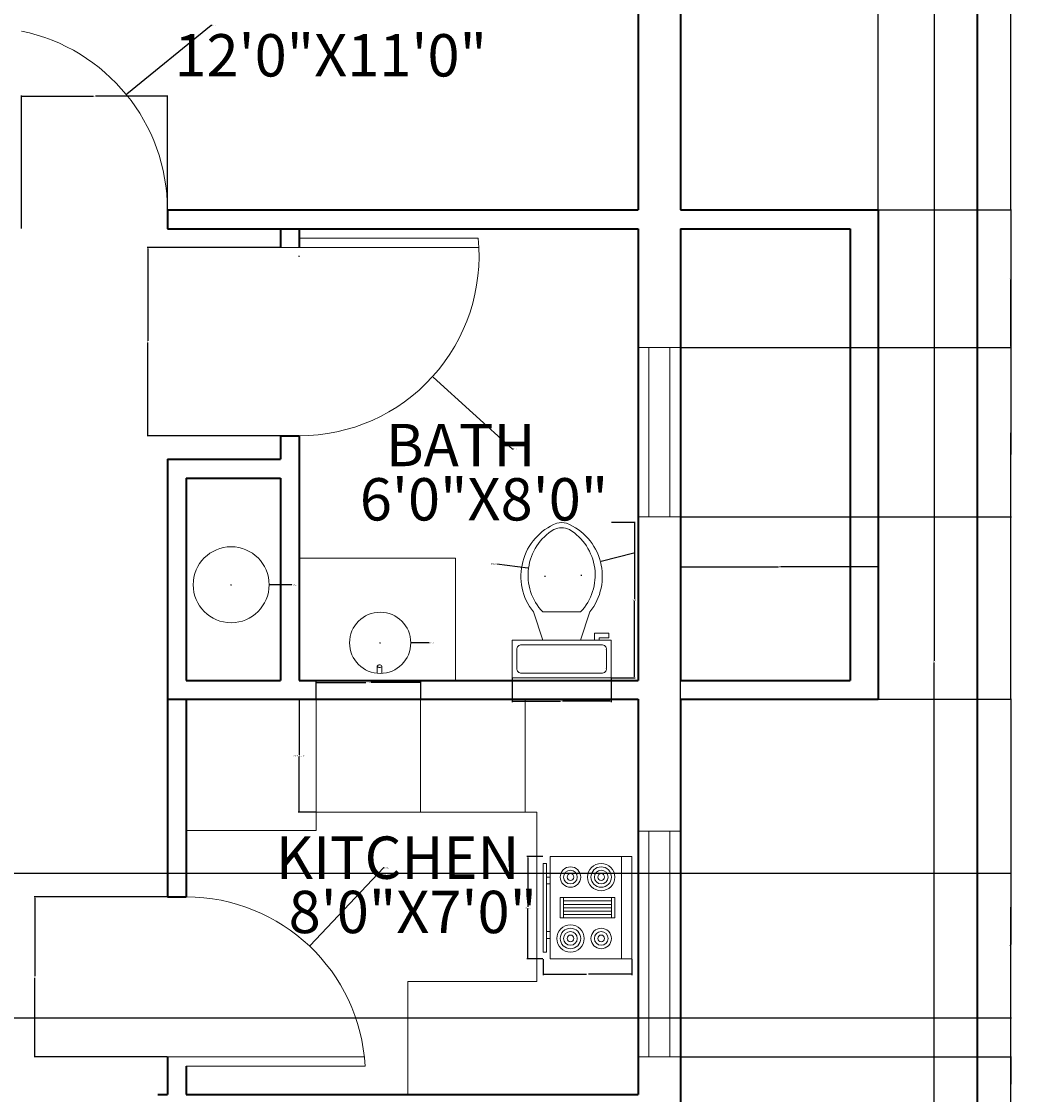
# Model space of a CAD drawing. Units: inches. Extents: x 1762 to 3150, y 1680 to 2382.
# Tile 3 of 6: x 1983 to 2199, y 1904 to 2132. Entities that reach past the tile are written whole.
import ezdxf

# ---------------------------------------------------------------- set-up
doc = ezdxf.new("R2010")
doc.units = ezdxf.units.IN
for name, color, linetype, lineweight in [('A-ANNO-DIMS', 2, 'Continuous', 18), ('A-ANNO-TTLB', 7, 'Continuous', 35), ('A-AREA-IDEN', 7, 'Continuous', 18), ('A-DOOR', 3, 'Continuous', 18), ('A-EQPM', 8, 'Continuous', 18), ('A-FLOR-FIXT', 9, 'Continuous', 18), ('A-GLAZ', 4, 'Continuous', 18), ('A-WALL', 7, 'Continuous', 35)]:
    doc.layers.add(name, color=color, linetype=linetype, lineweight=lineweight)
doc.layers.add('A-FLOR-CASE', color=242, linetype='Continuous', lineweight=18, true_color=0xcd2027)
doc.styles.get("Standard").update_dxf_attribs({"font": 'arial.ttf'})
doc.dimstyles.get("Standard").update_dxf_attribs({"dimtxt": 0.18, "dimasz": 0.18, "dimexe": 0.18, "dimexo": 0.0625, "dimgap": 0.09, "dimtad": 0, "dimtih": 1, "dimtoh": 1, "dimdec": 4, "dimzin": 0, "dimdsep": 46, "dimtxsty": 'Standard', "dimcen": 0.09, "dimadec": 0, "dimazin": 0, "dimtfac": 1, "dimtdec": 4, "dimtofl": 0, "dimtmove": 0, "dimatfit": 3, "dimfxl": 1, "dimtolj": 1, "dimtzin": 0, "dimarcsym": 0})

# ---------------------------------------------------------------- blocks, each defined once
blk = doc.blocks.new('Range-Oven - 30 in top')
for p, q in [((0, -3), (30, -3)), ((12, -6), (18, -6)), ((13, -20), (13, -6)), ((14, -6), (14, -20)), ((15, -20), (15, -6)), ((16, -6), (16, -20)), ((17, -20), (17, -6)), ((18, -20), (12, -20)), ((6, -24), (6, -25)), ((8, -25), (8, -24)), ((22, -25), (22, -24)), ((24, -24), (24, -25))]:
    blk.add_line(p, q)
for points in [[(0, -24), (0, 0), (30, 0), (30, -24)], [(12, -21), (12, -5), (18, -5), (18, -21)], [(2, -26), (2, -25), (28, -25), (28, -26)]]:
    blk.add_lwpolyline(points, close=True)
for centre, radius in [((6, -9), 4), ((6, -9), 3), ((24, -9), 3), ((6, -9), 2), ((6, -9), 1), ((24, -9), 2), ((24, -9), 1), ((6, -18), 3), ((24, -18), 4), ((24, -18), 3), ((6, -18), 2), ((6, -18), 1), ((24, -18), 2), ((24, -18), 1)]:
    blk.add_circle(centre, radius)
blk = doc.blocks.new('Toilet - top')
for p, q in [((9.5, -6), (9.5, -2)), ((-10, -8.5), (-8, -8.5)), ((-10, -9.5), (-10, -8.5)), ((-8, -8.5), (-8, -8)), ((-7, -8), (-7, -9.5)), ((-4, -8), (-6, -14)), ((4, -8), (6, -14)), ((-7, -9.5), (-10, -9.5)), ((4, -14), (-4, -14))]:
    blk.add_line(p, q)
blk.add_lwpolyline([(10.5, -8), (10.5, 0), (-10.5, 0), (-10.5, -8)], close=True)
for points in [[(-9.5, -2), (-9.5, -6)], [(8.5, -1), (-8.5, -1)], [(-8.5, -7), (8.5, -7)]]:
    blk.add_lwpolyline(points)
for centre, radius, start, end in [((-8.62, -1.88), 0.884, 81.8699, 188.1301), ((8.62, -1.88), 0.884, 351.8699, 98.1301), ((-8.62, -6.12), 0.884, 171.8699, 278.1301), ((8.62, -6.12), 0.884, 261.8699, 8.1301), ((3.52, -21.58), 12.17, 141.4691, 247.9714), ((4.2, -21.82), 11.33, 136.3677, 238.9468), ((-3.52, -21.58), 12.17, 292.0284, 38.5307), ((-4.2, -21.82), 11.33, 301.053, 43.6321), ((0, -27.88), 4, 245.7318, 294.2682), ((0, -29), 4, 254.8605, 285.1395)]:
    blk.add_arc(centre, radius, start, end)
blk = doc.blocks.new('WINDOW-48IN')
for p, q in [((0, 48), (9, 48)), ((2.25, 48), (2.25, 0)), ((6.75, 48), (6.75, 0)), ((0, 0), (9, 0))]:
    blk.add_line(p, q)
blk = doc.blocks.new('KITCHEN-BASE-MODULE')
blk.add_lwpolyline([(0, 24), (22.2, 24), (22.2, 0), (0, 0)], close=True)
blk = doc.blocks.new('*D24')
at = {"layer": 'A-ANNO-DIMS', "color": 0, "lineweight": -2, "transparency": 16777216}
for p, q in [((2045.07, 1987.99), (2041.35, 1987.99)), ((2041.53, 1987.81), (2041.53, 1976.17)), ((2041.53, 1964.17), (2041.53, 1975.81)), ((2045.07, 1963.99), (2041.35, 1963.99))]:
    blk.add_line(p, q, dxfattribs=at)
at = {"layer": 'A-ANNO-DIMS', "color": 0, "transparency": 16777216}
for points in [[(2041.5, 1987.81), (2041.56, 1987.81), (2041.53, 1987.99)], [(2041.5, 1964.17), (2041.56, 1964.17), (2041.53, 1963.99)]]:
    blk.add_solid(points, dxfattribs=at)
at = {"layer": 'Defpoints', "color": 0, "transparency": 16777216}
for p in [(2041.53, 1987.99), (2045.13, 1987.99), (2045.13, 1963.99)]:
    blk.add_point(p, dxfattribs=at)
at = {"layer": 'A-ANNO-DIMS', "color": 0, "transparency": 16777216, "insert": (2041.53, 1975.99), "char_height": 0.18, "attachment_point": 5}
blk.add_mtext('\\A1;BASE CABINET 24 TYP.', dxfattribs=at)
blk = doc.blocks.new('*D25')
at = {"layer": 'A-ANNO-DIMS', "color": 0, "lineweight": -2, "transparency": 16777216}
for p, q in [((2045.13, 1988.05), (2045.13, 1991.77)), ((2045.31, 1991.59), (2055.71, 1991.59)), ((2067.16, 1991.59), (2056.76, 1991.59)), ((2067.34, 1988.05), (2067.34, 1991.77))]:
    blk.add_line(p, q, dxfattribs=at)
at = {"layer": 'A-ANNO-DIMS', "color": 0, "transparency": 16777216}
for points in [[(2045.31, 1991.62), (2045.31, 1991.56), (2045.13, 1991.59)], [(2067.16, 1991.62), (2067.16, 1991.56), (2067.34, 1991.59)]]:
    blk.add_solid(points, dxfattribs=at)
at = {"layer": 'Defpoints', "color": 0, "transparency": 16777216}
for p in [(2067.34, 1991.59), (2045.13, 1987.99), (2067.34, 1987.99)]:
    blk.add_point(p, dxfattribs=at)
at = {"layer": 'A-ANNO-DIMS', "color": 0, "transparency": 16777216, "insert": (2056.24, 1991.59), "char_height": 0.18, "attachment_point": 5}
blk.add_mtext('\\A1;22 TYP.', dxfattribs=at)
blk = doc.blocks.new('*D26')
at = {"layer": 'A-ANNO-DIMS', "color": 0, "lineweight": -2, "transparency": 16777216}
for p, q in [((2107.84, 2025.6), (2112.91, 2025.6)), ((2112.73, 2025.42), (2112.73, 2009.26)), ((2112.73, 1992.73), (2112.73, 2008.89)), ((2107.84, 1992.55), (2112.91, 1992.55))]:
    blk.add_line(p, q, dxfattribs=at)
at = {"layer": 'A-ANNO-DIMS', "color": 0, "transparency": 16777216}
for points in [[(2112.7, 2025.42), (2112.76, 2025.42), (2112.73, 2025.6)], [(2112.7, 1992.73), (2112.76, 1992.73), (2112.73, 1992.55)]]:
    blk.add_solid(points, dxfattribs=at)
at = {"layer": 'Defpoints', "color": 0, "transparency": 16777216}
for p in [(2107.78, 2025.6), (2107.78, 1992.55), (2112.73, 1992.55)]:
    blk.add_point(p, dxfattribs=at)
at = {"layer": 'A-ANNO-DIMS', "color": 0, "transparency": 16777216, "insert": (2112.73, 2009.07), "char_height": 0.18, "attachment_point": 5}
blk.add_mtext('\\A1;WC 33', dxfattribs=at)
blk = doc.blocks.new('*D27')
at = {"layer": 'A-ANNO-DIMS', "color": 0, "lineweight": -2, "transparency": 16777216}
for p, q in [((2086.78, 1992.49), (2086.78, 1987.41)), ((2107.78, 1992.49), (2107.78, 1987.41)), ((2086.96, 1987.59), (2097.07, 1987.59)), ((2107.6, 1987.59), (2097.48, 1987.59))]:
    blk.add_line(p, q, dxfattribs=at)
at = {"layer": 'A-ANNO-DIMS', "color": 0, "transparency": 16777216}
for points in [[(2086.96, 1987.62), (2086.96, 1987.56), (2086.78, 1987.59)], [(2107.6, 1987.62), (2107.6, 1987.56), (2107.78, 1987.59)]]:
    blk.add_solid(points, dxfattribs=at)
at = {"layer": 'Defpoints', "color": 0, "transparency": 16777216}
for p in [(2086.78, 1992.55), (2107.78, 1992.55), (2086.78, 1987.59)]:
    blk.add_point(p, dxfattribs=at)
at = {"layer": 'A-ANNO-DIMS', "color": 0, "transparency": 16777216, "insert": (2097.28, 1987.59), "char_height": 0.18, "attachment_point": 5}
blk.add_mtext('\\A1;21', dxfattribs=at)
blk = doc.blocks.new('*D28')
at = {"layer": 'A-ANNO-DIMS', "color": 0, "lineweight": -2, "transparency": 16777216}
for p, q in [((2093.3, 1954.55), (2089.92, 1954.55)), ((2090.1, 1954.37), (2090.1, 1943.87)), ((2090.1, 1932.99), (2090.1, 1943.5)), ((2093.3, 1932.81), (2089.92, 1932.81))]:
    blk.add_line(p, q, dxfattribs=at)
at = {"layer": 'A-ANNO-DIMS', "color": 0, "transparency": 16777216}
for points in [[(2090.07, 1954.37), (2090.13, 1954.37), (2090.1, 1954.55)], [(2090.07, 1932.99), (2090.13, 1932.99), (2090.1, 1932.81)]]:
    blk.add_solid(points, dxfattribs=at)
at = {"layer": 'Defpoints', "color": 0, "transparency": 16777216}
for p in [(2093.36, 1954.55), (2090.1, 1932.81), (2093.36, 1932.81)]:
    blk.add_point(p, dxfattribs=at)
at = {"layer": 'A-ANNO-DIMS', "color": 0, "transparency": 16777216, "insert": (2090.1, 1943.68), "char_height": 0.18, "attachment_point": 5}
blk.add_mtext('\\A1;RANGE 22', dxfattribs=at)
blk = doc.blocks.new('*D29')
at = {"layer": 'A-ANNO-DIMS', "color": 0, "lineweight": -2, "transparency": 16777216}
for p, q in [((2093.36, 1932.75), (2093.36, 1929.37)), ((2112.21, 1932.75), (2112.21, 1929.37)), ((2093.54, 1929.55), (2102.57, 1929.55)), ((2112.03, 1929.55), (2103, 1929.55))]:
    blk.add_line(p, q, dxfattribs=at)
at = {"layer": 'A-ANNO-DIMS', "color": 0, "transparency": 16777216}
for points in [[(2093.54, 1929.58), (2093.54, 1929.52), (2093.36, 1929.55)], [(2112.03, 1929.58), (2112.03, 1929.52), (2112.21, 1929.55)]]:
    blk.add_solid(points, dxfattribs=at)
at = {"layer": 'Defpoints', "color": 0, "transparency": 16777216}
for p in [(2093.36, 1932.81), (2112.21, 1932.81), (2112.21, 1929.55)]:
    blk.add_point(p, dxfattribs=at)
at = {"layer": 'A-ANNO-DIMS', "color": 0, "transparency": 16777216, "insert": (2102.78, 1929.55), "char_height": 0.18, "attachment_point": 5}
blk.add_mtext('\\A1;19', dxfattribs=at)
blk = doc.blocks.new('*D32')
at = {"layer": 'A-ANNO-DIMS', "color": 0, "lineweight": -2, "transparency": 16777216}
for p, q in [((1846.54, 2121.05), (1846.54, 2325.32)), ((1846.72, 2325.14), (2005.25, 2325.14)), ((2164.36, 2325.14), (2005.83, 2325.14)), ((2164.54, 2092.05), (2164.54, 2325.32))]:
    blk.add_line(p, q, dxfattribs=at)
at = {"layer": 'A-ANNO-DIMS', "color": 0, "transparency": 16777216}
for points in [[(1846.72, 2325.17), (1846.72, 2325.11), (1846.54, 2325.14)], [(2164.36, 2325.17), (2164.36, 2325.11), (2164.54, 2325.14)]]:
    blk.add_solid(points, dxfattribs=at)
at = {"layer": 'Defpoints', "color": 0, "transparency": 16777216}
for p in [(2164.54, 2325.14), (1846.54, 2120.99), (2164.54, 2091.99)]:
    blk.add_point(p, dxfattribs=at)
at = {"layer": 'A-ANNO-DIMS', "color": 0, "transparency": 16777216, "insert": (2005.54, 2325.14), "char_height": 0.18, "attachment_point": 5}
blk.add_mtext('\\A1;318', dxfattribs=at)
blk = doc.blocks.new('*D36')
at = {"layer": 'A-ANNO-DIMS', "color": 0, "lineweight": -2, "transparency": 16777216}
for p, q in [((2164.6, 1987.99), (2192.87, 1987.99)), ((2192.69, 1987.81), (2192.69, 1944.17)), ((2192.69, 1900.17), (2192.69, 1943.81)), ((2122.6, 1899.99), (2192.87, 1899.99))]:
    blk.add_line(p, q, dxfattribs=at)
at = {"layer": 'A-ANNO-DIMS', "color": 0, "transparency": 16777216}
for points in [[(2192.66, 1987.81), (2192.72, 1987.81), (2192.69, 1987.99)], [(2192.66, 1900.17), (2192.72, 1900.17), (2192.69, 1899.99)]]:
    blk.add_solid(points, dxfattribs=at)
at = {"layer": 'Defpoints', "color": 0, "transparency": 16777216}
for p in [(2164.54, 1987.99), (2192.69, 1987.99), (2122.54, 1899.99)]:
    blk.add_point(p, dxfattribs=at)
at = {"layer": 'A-ANNO-DIMS', "color": 0, "transparency": 16777216, "insert": (2192.69, 1943.99), "char_height": 0.18, "attachment_point": 5}
blk.add_mtext('\\A1;88', dxfattribs=at)
blk = doc.blocks.new('*D37')
at = {"layer": 'A-ANNO-DIMS', "color": 0, "lineweight": -2, "transparency": 16777216}
for p, q in [((2164.6, 2091.99), (2192.87, 2091.99)), ((2192.69, 2091.81), (2192.69, 2040.17)), ((2192.69, 1988.17), (2192.69, 2039.81)), ((2164.6, 1987.99), (2192.87, 1987.99))]:
    blk.add_line(p, q, dxfattribs=at)
at = {"layer": 'A-ANNO-DIMS', "color": 0, "transparency": 16777216}
for points in [[(2192.66, 2091.81), (2192.72, 2091.81), (2192.69, 2091.99)], [(2192.66, 1988.17), (2192.72, 1988.17), (2192.69, 1987.99)]]:
    blk.add_solid(points, dxfattribs=at)
at = {"layer": 'Defpoints', "color": 0, "transparency": 16777216}
for p in [(2164.54, 2091.99), (2192.69, 2091.99), (2164.54, 1987.99)]:
    blk.add_point(p, dxfattribs=at)
at = {"layer": 'A-ANNO-DIMS', "color": 0, "transparency": 16777216, "insert": (2192.69, 2039.99), "char_height": 0.18, "attachment_point": 5}
blk.add_mtext('\\A1;104', dxfattribs=at)
blk = doc.blocks.new('*D38')
at = {"layer": 'A-ANNO-DIMS', "color": 0, "lineweight": -2, "transparency": 16777216}
for p, q in [((2122.6, 2232.99), (2192.87, 2232.99)), ((2192.69, 2232.81), (2192.69, 2162.67)), ((2192.69, 2092.17), (2192.69, 2162.31)), ((2164.6, 2091.99), (2192.87, 2091.99))]:
    blk.add_line(p, q, dxfattribs=at)
at = {"layer": 'A-ANNO-DIMS', "color": 0, "transparency": 16777216}
for points in [[(2192.66, 2232.81), (2192.72, 2232.81), (2192.69, 2232.99)], [(2192.66, 2092.17), (2192.72, 2092.17), (2192.69, 2091.99)]]:
    blk.add_solid(points, dxfattribs=at)
at = {"layer": 'Defpoints', "color": 0, "transparency": 16777216}
for p in [(2122.54, 2232.99), (2192.69, 2232.99), (2164.54, 2091.99)]:
    blk.add_point(p, dxfattribs=at)
at = {"layer": 'A-ANNO-DIMS', "color": 0, "transparency": 16777216, "insert": (2192.69, 2162.49), "char_height": 0.18, "attachment_point": 5}
blk.add_mtext('\\A1;141', dxfattribs=at)
blk = doc.blocks.new('*D43')
at = {"layer": 'A-ANNO-DIMS', "color": 0, "lineweight": -2, "transparency": 16777216}
for p, q in [((2122.54, 1988.05), (2122.54, 2016.32)), ((2122.72, 2016.14), (2143.32, 2016.14)), ((2164.36, 2016.14), (2143.76, 2016.14)), ((2164.54, 1988.05), (2164.54, 2016.32))]:
    blk.add_line(p, q, dxfattribs=at)
at = {"layer": 'A-ANNO-DIMS', "color": 0, "transparency": 16777216}
for points in [[(2122.72, 2016.17), (2122.72, 2016.11), (2122.54, 2016.14)], [(2164.36, 2016.17), (2164.36, 2016.11), (2164.54, 2016.14)]]:
    blk.add_solid(points, dxfattribs=at)
at = {"layer": 'Defpoints', "color": 0, "transparency": 16777216}
for p in [(2164.54, 2016.14), (2122.54, 1987.99), (2164.54, 1987.99)]:
    blk.add_point(p, dxfattribs=at)
at = {"layer": 'A-ANNO-DIMS', "color": 0, "transparency": 16777216, "insert": (2143.54, 2016.14), "char_height": 0.18, "attachment_point": 5}
blk.add_mtext('\\A1;42', dxfattribs=at)
blk = doc.blocks.new('*D49')
at = {"layer": 'A-ANNO-DIMS', "color": 0, "lineweight": -2, "transparency": 16777216}
for p, q in [((1982.54, 2088.05), (1982.54, 2116.32)), ((1982.72, 2116.14), (1997.84, 2116.14)), ((2013.36, 2116.14), (1998.24, 2116.14)), ((2013.54, 2088.05), (2013.54, 2116.32))]:
    blk.add_line(p, q, dxfattribs=at)
at = {"layer": 'A-ANNO-DIMS', "color": 0, "transparency": 16777216}
for points in [[(1982.72, 2116.17), (1982.72, 2116.11), (1982.54, 2116.14)], [(2013.36, 2116.17), (2013.36, 2116.11), (2013.54, 2116.14)]]:
    blk.add_solid(points, dxfattribs=at)
at = {"layer": 'Defpoints', "color": 0, "transparency": 16777216}
for p in [(2013.54, 2116.14), (1982.54, 2087.99), (2013.54, 2087.99)]:
    blk.add_point(p, dxfattribs=at)
at = {"layer": 'A-ANNO-DIMS', "color": 0, "transparency": 16777216, "insert": (1998.04, 2116.14), "char_height": 0.18, "attachment_point": 5}
blk.add_mtext('\\A1;31', dxfattribs=at)
blk = doc.blocks.new('*D52')
at = {"layer": 'A-ANNO-DIMS', "color": 0, "lineweight": -2, "transparency": 16777216}
for p, q in [((2037.48, 2083.99), (2009.21, 2083.99)), ((2009.39, 2083.81), (2009.39, 2064.17)), ((2009.39, 2044.17), (2009.39, 2063.81)), ((2037.48, 2043.99), (2009.21, 2043.99))]:
    blk.add_line(p, q, dxfattribs=at)
at = {"layer": 'A-ANNO-DIMS', "color": 0, "transparency": 16777216}
for points in [[(2009.36, 2083.81), (2009.42, 2083.81), (2009.39, 2083.99)], [(2009.36, 2044.17), (2009.42, 2044.17), (2009.39, 2043.99)]]:
    blk.add_solid(points, dxfattribs=at)
at = {"layer": 'Defpoints', "color": 0, "transparency": 16777216}
for p in [(2009.39, 2083.99), (2037.54, 2083.99), (2037.54, 2043.99)]:
    blk.add_point(p, dxfattribs=at)
at = {"layer": 'A-ANNO-DIMS', "color": 0, "transparency": 16777216, "insert": (2009.39, 2063.99), "char_height": 0.18, "attachment_point": 5}
blk.add_mtext('\\A1;40', dxfattribs=at)
blk = doc.blocks.new('*D53')
at = {"layer": 'A-ANNO-DIMS', "color": 0, "lineweight": -2, "transparency": 16777216}
for p, q in [((2013.48, 1945.99), (1985.21, 1945.99)), ((1985.39, 1945.81), (1985.39, 1929.17)), ((1985.39, 1912.17), (1985.39, 1928.81)), ((2013.48, 1911.99), (1985.21, 1911.99))]:
    blk.add_line(p, q, dxfattribs=at)
at = {"layer": 'A-ANNO-DIMS', "color": 0, "transparency": 16777216}
for points in [[(1985.36, 1945.81), (1985.42, 1945.81), (1985.39, 1945.99)], [(1985.36, 1912.17), (1985.42, 1912.17), (1985.39, 1911.99)]]:
    blk.add_solid(points, dxfattribs=at)
at = {"layer": 'Defpoints', "color": 0, "transparency": 16777216}
for p in [(1985.39, 1945.99), (2013.54, 1945.99), (2013.54, 1911.99)]:
    blk.add_point(p, dxfattribs=at)
at = {"layer": 'A-ANNO-DIMS', "color": 0, "transparency": 16777216, "insert": (1985.39, 1928.99), "char_height": 0.18, "attachment_point": 5}
blk.add_mtext('\\A1;34', dxfattribs=at)
blk = doc.blocks.new('*D54')
at = {"layer": 'A-ANNO-DIMS', "color": 0, "lineweight": -2, "transparency": 16777216}
for p, q in [((2122.6, 2062.78), (2192.87, 2062.78)), ((2192.69, 2062.6), (2192.69, 2044.96)), ((2192.69, 2026.96), (2192.69, 2044.6)), ((2122.6, 2026.78), (2192.87, 2026.78))]:
    blk.add_line(p, q, dxfattribs=at)
at = {"layer": 'A-ANNO-DIMS', "color": 0, "transparency": 16777216}
for points in [[(2192.66, 2062.6), (2192.72, 2062.6), (2192.69, 2062.78)], [(2192.66, 2026.96), (2192.72, 2026.96), (2192.69, 2026.78)]]:
    blk.add_solid(points, dxfattribs=at)
at = {"layer": 'Defpoints', "color": 0, "transparency": 16777216}
for p in [(2122.54, 2062.78), (2192.69, 2062.78), (2122.54, 2026.78)]:
    blk.add_point(p, dxfattribs=at)
at = {"layer": 'A-ANNO-DIMS', "color": 0, "transparency": 16777216, "insert": (2192.69, 2044.78), "char_height": 0.18, "attachment_point": 5}
blk.add_mtext('\\A1;36', dxfattribs=at)
blk = doc.blocks.new('*D55')
at = {"layer": 'A-ANNO-DIMS', "color": 0, "lineweight": -2, "transparency": 16777216}
for p, q in [((2122.6, 2091.99), (2192.87, 2091.99)), ((2192.69, 2091.81), (2192.69, 2077.57)), ((2192.69, 2062.96), (2192.69, 2077.2)), ((2122.6, 2062.78), (2192.87, 2062.78))]:
    blk.add_line(p, q, dxfattribs=at)
at = {"layer": 'A-ANNO-DIMS', "color": 0, "transparency": 16777216}
for points in [[(2192.66, 2091.81), (2192.72, 2091.81), (2192.69, 2091.99)], [(2192.66, 2062.96), (2192.72, 2062.96), (2192.69, 2062.78)]]:
    blk.add_solid(points, dxfattribs=at)
at = {"layer": 'Defpoints', "color": 0, "transparency": 16777216}
for p in [(2122.54, 2091.99), (2192.69, 2091.99), (2122.54, 2062.78)]:
    blk.add_point(p, dxfattribs=at)
at = {"layer": 'A-ANNO-DIMS', "color": 0, "transparency": 16777216, "insert": (2192.69, 2077.39), "char_height": 0.18, "attachment_point": 5}
blk.add_mtext('\\A1;29.21', dxfattribs=at)
blk = doc.blocks.new('*D56')
at = {"layer": 'A-ANNO-DIMS', "color": 0, "lineweight": -2, "transparency": 16777216}
for p, q in [((2122.6, 1911.99), (2192.87, 1911.99)), ((2192.69, 1911.81), (2192.69, 1906.17)), ((2192.69, 1900.17), (2192.69, 1905.81)), ((2122.6, 1899.99), (2192.87, 1899.99))]:
    blk.add_line(p, q, dxfattribs=at)
at = {"layer": 'A-ANNO-DIMS', "color": 0, "transparency": 16777216}
for points in [[(2192.66, 1911.81), (2192.72, 1911.81), (2192.69, 1911.99)], [(2192.66, 1900.17), (2192.72, 1900.17), (2192.69, 1899.99)]]:
    blk.add_solid(points, dxfattribs=at)
at = {"layer": 'Defpoints', "color": 0, "transparency": 16777216}
for p in [(2122.54, 1911.99), (2192.69, 1911.99), (2122.54, 1899.99)]:
    blk.add_point(p, dxfattribs=at)
at = {"layer": 'A-ANNO-DIMS', "color": 0, "transparency": 16777216, "insert": (2192.69, 1905.99), "char_height": 0.18, "attachment_point": 5}
blk.add_mtext('\\A1;12', dxfattribs=at)
blk = doc.blocks.new('*D58')
at = {"layer": 'A-ANNO-DIMS', "color": 0, "lineweight": -2, "transparency": 16777216}
for p, q in [((1964.15, 1951.05), (2192.87, 1951.05)), ((2192.69, 1950.87), (2192.69, 1935.87)), ((2192.69, 1920.49), (2192.69, 1935.5)), ((1964.15, 1920.31), (2192.87, 1920.31))]:
    blk.add_line(p, q, dxfattribs=at)
at = {"layer": 'A-ANNO-DIMS', "color": 0, "transparency": 16777216}
for points in [[(2192.66, 1950.87), (2192.72, 1950.87), (2192.69, 1951.05)], [(2192.66, 1920.49), (2192.72, 1920.49), (2192.69, 1920.31)]]:
    blk.add_solid(points, dxfattribs=at)
at = {"layer": 'Defpoints', "color": 0, "transparency": 16777216}
for p in [(1964.09, 1951.05), (1964.09, 1920.31), (2192.69, 1920.31)]:
    blk.add_point(p, dxfattribs=at)
at = {"layer": 'A-ANNO-DIMS', "color": 0, "transparency": 16777216, "insert": (2192.69, 1935.68), "char_height": 0.18, "attachment_point": 5}
blk.add_mtext('\\A1;30.74', dxfattribs=at)
blk = doc.blocks.new('*D65')
at = {"layer": 'A-ANNO-DIMS', "color": 0, "lineweight": -2, "transparency": 16777216}
for p, q in [((2364.876105, 2232.98945), (2176.268936, 2232.98945)), ((2176.448936, 2232.80945), (2176.448936, 1996.16945)), ((2176.448936, 1759.16945), (2176.448936, 1995.80945)), ((2239.876105, 1758.98945), (2176.268936, 1758.98945))]:
    blk.add_line(p, q, dxfattribs=at)
at = {"layer": 'A-ANNO-DIMS', "color": 0, "transparency": 16777216}
for points in [[(2176.418936, 2232.80945), (2176.478936, 2232.80945), (2176.448936, 2232.98945)], [(2176.418936, 1759.16945), (2176.478936, 1759.16945), (2176.448936, 1758.98945)]]:
    blk.add_solid(points, dxfattribs=at)
at = {"layer": 'Defpoints', "color": 0, "transparency": 16777216}
for p in [(2176.448936, 2232.98945), (2364.938605, 2232.98945), (2239.938605, 1758.98945)]:
    blk.add_point(p, dxfattribs=at)
at = {"layer": 'A-ANNO-DIMS', "color": 0, "transparency": 16777216, "insert": (2176.448936, 1995.98945), "char_height": 0.18, "attachment_point": 5}
blk.add_mtext('\\A1;474', dxfattribs=at)
blk = doc.blocks.new('*D99')
at = {"layer": 'A-ANNO-DIMS', "color": 0, "lineweight": -2, "transparency": 16777216}
for p, q in [((2022.84, 2131.22), (2004.94, 2116.62)), ((2023.02, 2131.22), (2022.84, 2131.22)), ((1974.66, 2091.99), (1974.84, 2091.99)), ((1974.75, 2091.9), (1974.75, 2092.08))]:
    blk.add_line(p, q, dxfattribs=at)
at = {"layer": 'A-ANNO-DIMS', "color": 0, "transparency": 16777216}
blk.add_solid([(2004.93, 2116.65), (2004.96, 2116.6), (2004.81, 2116.51)], dxfattribs=at)
at = {"layer": 'Defpoints', "color": 0, "transparency": 16777216}
for p in [(2004.81, 2116.51), (1974.75, 2091.99)]:
    blk.add_point(p, dxfattribs=at)
at = {"layer": 'A-ANNO-DIMS', "color": 0, "transparency": 16777216, "insert": (2023.5, 2131.22), "char_height": 0.18, "attachment_point": 5}
blk.add_mtext('\\A1;R38.79', dxfattribs=at)
blk = doc.blocks.new('*D100')
at = {"layer": 'A-ANNO-DIMS', "color": 0, "lineweight": -2, "transparency": 16777216}
for p, q in [((2041.45, 2082.18), (2041.63, 2082.18)), ((2041.54, 2082.09), (2041.54, 2082.27)), ((2086.85, 2041.18), (2069.99, 2056.44)), ((2087.03, 2041.18), (2086.85, 2041.18))]:
    blk.add_line(p, q, dxfattribs=at)
at = {"layer": 'A-ANNO-DIMS', "color": 0, "transparency": 16777216}
blk.add_solid([(2070.01, 2056.46), (2069.97, 2056.41), (2069.86, 2056.56)], dxfattribs=at)
at = {"layer": 'Defpoints', "color": 0, "transparency": 16777216}
for p in [(2041.54, 2082.18), (2069.86, 2056.56)]:
    blk.add_point(p, dxfattribs=at)
at = {"layer": 'A-ANNO-DIMS', "color": 0, "transparency": 16777216, "insert": (2087.51, 2041.18), "char_height": 0.18, "attachment_point": 5}
blk.add_mtext('\\A1;R38.19', dxfattribs=at)
blk = doc.blocks.new('*D101')
at = {"layer": 'A-ANNO-DIMS', "color": 0, "lineweight": -2, "transparency": 16777216}
for p, q in [((2059.41, 1952.14), (2043.83, 1935.69)), ((2059.59, 1952.14), (2059.41, 1952.14)), ((2017.45, 1907.93), (2017.63, 1907.93)), ((2017.54, 1907.84), (2017.54, 1908.02))]:
    blk.add_line(p, q, dxfattribs=at)
at = {"layer": 'A-ANNO-DIMS', "color": 0, "transparency": 16777216}
blk.add_solid([(2043.81, 1935.71), (2043.86, 1935.67), (2043.71, 1935.56)], dxfattribs=at)
at = {"layer": 'Defpoints', "color": 0, "transparency": 16777216}
for p in [(2043.71, 1935.56), (2017.54, 1907.93)]:
    blk.add_point(p, dxfattribs=at)
at = {"layer": 'A-ANNO-DIMS', "color": 0, "transparency": 16777216, "insert": (2060.14, 1952.14), "char_height": 0.18, "attachment_point": 5}
blk.add_mtext('\\A1;R38.056', dxfattribs=at)
blk = doc.blocks.new('*D103')
at = {"layer": 'A-ANNO-DIMS', "color": 0, "lineweight": -2, "transparency": 16777216}
for p, q in [((2026.99, 2012.33), (2027.17, 2012.33)), ((2027.08, 2012.24), (2027.08, 2012.42)), ((2039.99, 2012.33), (2035.33, 2012.33))]:
    blk.add_line(p, q, dxfattribs=at)
at = {"layer": 'A-ANNO-DIMS', "color": 0, "transparency": 16777216}
blk.add_solid([(2035.33, 2012.36), (2035.33, 2012.3), (2035.15, 2012.33)], dxfattribs=at)
at = {"layer": 'Defpoints', "color": 0, "transparency": 16777216}
for p in [(2019.01, 2012.33), (2035.15, 2012.33)]:
    blk.add_point(p, dxfattribs=at)
at = {"layer": 'A-ANNO-DIMS', "color": 0, "transparency": 16777216, "insert": (2040.55, 2012.33), "char_height": 0.18, "attachment_point": 5}
blk.add_mtext('\\A1;∅16.138', dxfattribs=at)
blk = doc.blocks.new('*D104')
at = {"layer": 'A-ANNO-DIMS', "color": 0, "lineweight": -2, "transparency": 16777216}
for p, q in [((2058.74, 1999.9), (2058.74, 2000.08)), ((2058.65, 1999.99), (2058.83, 1999.99)), ((2069.15, 1999.99), (2065.42, 1999.99))]:
    blk.add_line(p, q, dxfattribs=at)
at = {"layer": 'A-ANNO-DIMS', "color": 0, "transparency": 16777216}
blk.add_solid([(2065.42, 2000.02), (2065.42, 1999.96), (2065.24, 1999.99)], dxfattribs=at)
at = {"layer": 'Defpoints', "color": 0, "transparency": 16777216}
for p in [(2052.23, 1999.99), (2065.24, 1999.99)]:
    blk.add_point(p, dxfattribs=at)
at = {"layer": 'A-ANNO-DIMS', "color": 0, "transparency": 16777216, "insert": (2069.62, 1999.99), "char_height": 0.18, "attachment_point": 5}
blk.add_mtext('\\A1;∅13.01', dxfattribs=at)
blk = doc.blocks.new('*D105')
at = {"layer": 'A-ANNO-DIMS', "color": 0, "lineweight": -2, "transparency": 16777216}
for p, q in [((2112.59, 2019.08), (2105.7, 2017.27)), ((2093.67, 2014.13), (2093.85, 2014.13)), ((2093.76, 2014.04), (2093.76, 2014.22))]:
    blk.add_line(p, q, dxfattribs=at)
at = {"layer": 'A-ANNO-DIMS', "color": 0, "transparency": 16777216}
blk.add_solid([(2105.69, 2017.3), (2105.71, 2017.24), (2105.53, 2017.22)], dxfattribs=at)
at = {"layer": 'Defpoints', "color": 0, "transparency": 16777216}
for p in [(2105.53, 2017.22), (2093.76, 2014.13)]:
    blk.add_point(p, dxfattribs=at)
at = {"layer": 'A-ANNO-DIMS', "color": 0, "transparency": 16777216, "insert": (2113.26, 2019.08), "char_height": 0.18, "attachment_point": 5}
blk.add_mtext('\\A1;2X R12.17', dxfattribs=at)
blk = doc.blocks.new('*D106')
at = {"layer": 'A-ANNO-DIMS', "color": 0, "lineweight": -2, "transparency": 16777216}
for p, q in [((2083.51, 2016.78), (2090.07, 2015.9)), ((2101.39, 2014.37), (2101.57, 2014.37)), ((2101.48, 2014.28), (2101.48, 2014.46))]:
    blk.add_line(p, q, dxfattribs=at)
at = {"layer": 'A-ANNO-DIMS', "color": 0, "transparency": 16777216}
blk.add_solid([(2090.07, 2015.93), (2090.07, 2015.87), (2090.25, 2015.88)], dxfattribs=at)
at = {"layer": 'Defpoints', "color": 0, "transparency": 16777216}
for p in [(2090.25, 2015.88), (2101.48, 2014.37)]:
    blk.add_point(p, dxfattribs=at)
at = {"layer": 'A-ANNO-DIMS', "color": 0, "transparency": 16777216, "insert": (2082.84, 2016.78), "char_height": 0.18, "attachment_point": 5}
blk.add_mtext('\\A1;2X R11.33', dxfattribs=at)

msp = doc.modelspace()

# ---------------------------------------------------------------- linework, layer by layer
at = {"layer": 'A-ANNO-TTLB'}
msp.add_line((2185.5413, 2359.5805), (2185.5413, 1709.6712), dxfattribs=at)
at = {"layer": 'A-DOOR'}
for p, q in [((2041.5385, 2085.9895), (2079.5385, 2085.9895)), ((2037.5385, 2083.9895), (2079.5385, 2083.9895)), ((2013.5385, 1911.9895), (2055.3773, 1911.9895)), ((2017.5385, 1909.9895), (2055.5385, 1909.9895))]:
    msp.add_line(p, q, dxfattribs=at)
for centre, radius, start, end in [((1974.7481, 2091.9894), 38.7903, 360, 78.414407), ((2041.5385, 2082.1799), 38.1905, 270, 5.72481), ((2017.5385, 1907.9339), 38.0556, 3.096315, 90)]:
    msp.add_arc(centre, radius, start, end, dxfattribs=at)
at = {"layer": 'A-FLOR-CASE'}
for p, q in [((2045.1342, 1963.9895), (2089.5385, 1963.9895)), ((2089.5385, 1963.9895), (2092.0017, 1963.9895)), ((2092.0017, 1963.9895), (2092.0017, 1927.9895)), ((2064.5921, 1927.9895), (2092.0017, 1927.9895)), ((2064.5921, 1927.9895), (2064.5921, 1903.9895))]:
    msp.add_line(p, q, dxfattribs=at)
msp.add_lwpolyline([(2017.5385, 1987.9895), (2045.1342, 1987.9895), (2045.1342, 1960.0721), (2017.5385, 1960.0721)], close=True, dxfattribs=at)
at = {"layer": 'A-FLOR-FIXT'}
for p, q in [((2041.5385, 2017.9895), (2074.7029, 2017.9895)), ((2074.7029, 2017.9895), (2074.7029, 1991.9895)), ((2058.1173, 1995.0309), (2058.1173, 1993.5766)), ((2059.1173, 1995.0309), (2059.1173, 1993.5766))]:
    msp.add_line(p, q, dxfattribs=at)
for centre, radius in [((2027.0819, 2012.3302), 8.0692), ((2058.7374, 1999.9931), 6.505)]:
    msp.add_circle(centre, radius, dxfattribs=at)
for centre, start, end in [((2058.6173, 1994.7466), 29.622214, 150.377786), ((2058.6173, 1995.3152), 209.622214, 330.377786)]:
    msp.add_arc(centre, 0.5752, start, end, dxfattribs=at)
at = {"layer": 'A-GLAZ'}
for p, q in [((2113.5385, 2062.7811), (2122.5385, 2062.7811)), ((2115.7885, 2062.7811), (2115.7885, 2026.7811)), ((2120.2885, 2062.7811), (2120.2885, 2026.7811)), ((2113.5385, 2026.7811), (2122.5385, 2026.7811))]:
    msp.add_line(p, q, dxfattribs=at)
at = {"layer": 'A-WALL'}
for p, q in [((2122.5385, 2232.9895), (2122.5385, 2091.9894)), ((2113.5385, 2223.9895), (2113.5385, 2091.9894)), ((2013.5385, 2091.9894), (2013.5385, 2087.9895)), ((2013.5385, 2091.9894), (2113.5385, 2091.9894)), ((2122.5385, 2091.9894), (2164.5385, 2091.9894)), ((2164.5385, 2091.9894), (2164.5385, 1987.9895)), ((2013.5385, 2087.9895), (2113.5385, 2087.9895)), ((2037.5385, 2087.9895), (2037.5385, 2083.9895)), ((2041.5385, 2087.9895), (2041.5385, 2083.9895)), ((2113.5385, 2087.9895), (2113.5385, 1991.9895)), ((2122.5385, 2087.9895), (2122.5385, 1991.9895)), ((2122.5385, 2087.9895), (2158.5385, 2087.9895)), ((2158.5385, 2087.9895), (2158.5385, 1991.9895)), ((2037.5385, 2043.9895), (2037.5385, 2038.9895)), ((2037.5385, 2043.9895), (2041.5385, 2043.9895)), ((2041.5385, 2043.9895), (2041.5385, 1991.9895)), ((2013.5385, 2038.9895), (2013.5385, 1945.9895)), ((2013.5385, 2038.9895), (2037.5385, 2038.9895)), ((2017.5385, 2034.9895), (2037.5385, 2034.9895)), ((2017.5385, 2034.9895), (2017.5385, 1991.9895)), ((2037.5385, 2034.9895), (2037.5385, 1991.9895)), ((2017.5385, 1991.9895), (2037.5385, 1991.9895)), ((2041.5385, 1991.9895), (2113.5385, 1991.9895)), ((2122.5385, 1991.9895), (2158.5385, 1991.9895)), ((2013.5385, 1987.9895), (2113.5385, 1987.9895)), ((2017.5385, 1987.9895), (2017.5385, 1945.9895)), ((2113.5385, 1987.9895), (2113.5385, 1903.9895)), ((2122.5385, 1987.9895), (2164.5385, 1987.9895)), ((2122.5385, 1987.9895), (2122.5385, 1899.9895)), ((2013.5385, 1945.9895), (2017.5385, 1945.9895)), ((2013.5385, 1911.9895), (2013.5385, 1903.9895)), ((2017.5385, 1909.9895), (2017.5385, 1903.9895)), ((2011.5385, 1903.9895), (2013.5385, 1903.9895)), ((2017.5385, 1903.9895), (2113.5385, 1903.9895))]:
    msp.add_line(p, q, dxfattribs=at)

# ---------------------------------------------------------------- block references
at = {"layer": 'A-EQPM', "xscale": 0.7246798212194462, "yscale": 0.7246798212194462, "zscale": 0.7246798212194462, "rotation": 270}
msp.add_blockref('Range-Oven - 30 in top', (2112.2056, 1954.5543), dxfattribs=at)
at = {"layer": 'A-FLOR-CASE'}
for p in [(2045.134, 1963.989), (2067.3361, 1963.989)]:
    msp.add_blockref('KITCHEN-BASE-MODULE', p, dxfattribs=at)
at = {"layer": 'A-FLOR-FIXT', "rotation": 180}
msp.add_blockref('Toilet - top', (2097.2767, 1992.5518), dxfattribs=at)
at = {"layer": 'A-GLAZ', "rotation": 180}
msp.add_blockref('WINDOW-48IN', (2122.5389, 1959.9899), dxfattribs=at)

# ---------------------------------------------------------------- texts
at = {"layer": 'A-AREA-IDEN'}
for s, p in [(' 12\'0"X11\'0"', (2012.2793, 2120.3527)), ('      BATH', (2043.4122, 2037.531)), ('    6\'0"X8\'0"', (2043.4122, 2025.9919)), ('KITCHEN', (2036.5397, 1949.8323)), (' 8\'0"X7\'0"', (2036.5397, 1938.2932))]:
    msp.add_text(s, height=9, dxfattribs=at).set_placement(p)

# ---------------------------------------------------------------- dimensions: what is measured, and where the dimension line sits
at = {"layer": 'A-ANNO-DIMS'}
for base, p1, p2, picture, middle in [((2164.5385, 2325.1356), (1846.5385, 2120.9895), (2164.5385, 2091.9894), '*D32', (2005.5385, 2325.1356)), ((2013.5385, 2116.1395), (1982.5385, 2087.9895), (2013.5385, 2087.9895), '*D49', (1998.0385, 2116.1395)), ((2164.5385, 2016.1394), (2122.5385, 1987.9895), (2164.5385, 1987.9895), '*D43', (2143.5385, 2016.1394)), ((2112.2056, 1929.5528), (2093.3639, 1932.8139), (2112.2056, 1932.8139), '*D29', (2102.7848, 1929.5528))]:
    dim = msp.add_linear_dim(base=base, p1=p1, p2=p2, dimstyle='Standard', override={"dimdec": 0, "dimlfac": 1, "dimrnd": 0, "dimzin": 0, "dimdsep": 46, "dimlunit": 2}, dxfattribs=at)
    dim.commit()
    dim.dimension.update_dxf_attribs({"geometry": picture, "text_midpoint": middle})
for base, p1, p2, angle, override, picture, middle in [((2192.6885, 2232.9895), (2164.5385, 2091.9894), (2122.5385, 2232.9895), 90, {"dimdec": 0, "dimlfac": 1, "dimrnd": 0, "dimzin": 0, "dimdsep": 46, "dimlunit": 2}, '*D38', (2192.6885, 2162.4895)), ((2176.4489, 2232.9895), (2239.9386, 1758.9895), (2364.9386, 2232.9895), 90, {"dimdec": 0, "dimlfac": 1, "dimrnd": 0, "dimzin": 0, "dimdsep": 46, "dimlunit": 2}, '*D65', (2176.4489, 1995.9894)), ((2192.6885, 2091.9894), (2122.5385, 2062.7811), (2122.5385, 2091.9894), 90, {"dimdec": 2, "dimlfac": 1, "dimrnd": 0, "dimzin": 0, "dimdsep": 46, "dimlunit": 2}, '*D55', (2192.6885, 2077.3853)), ((2192.6885, 2091.9894), (2164.5385, 1987.9895), (2164.5385, 2091.9894), 90, {"dimdec": 0, "dimlfac": 1, "dimrnd": 0, "dimzin": 0, "dimdsep": 46, "dimlunit": 2}, '*D37', (2192.6885, 2039.9895)), ((2009.3885, 2083.9895), (2037.5385, 2043.9895), (2037.5385, 2083.9895), 90, {"dimdec": 0, "dimlfac": 1, "dimrnd": 0, "dimzin": 0, "dimdsep": 46, "dimlunit": 2}, '*D52', (2009.3885, 2063.9895)), ((2192.6885, 2062.7811), (2122.5385, 2026.7811), (2122.5385, 2062.7811), 90, {"dimdec": 0, "dimlfac": 1, "dimrnd": 0, "dimzin": 0, "dimdsep": 46, "dimlunit": 2}, '*D54', (2192.6885, 2044.7811)), ((2086.7767, 1987.5949), (2107.7767, 1992.5518), (2086.7767, 1992.5518), 180, {"dimdec": 0, "dimlfac": 1, "dimrnd": 0, "dimzin": 0, "dimdsep": 46, "dimlunit": 2}, '*D27', (2097.2767, 1987.5949)), ((2192.6885, 1987.9895), (2122.5385, 1899.9895), (2164.5385, 1987.9895), 90, {"dimdec": 0, "dimlfac": 1, "dimrnd": 0, "dimzin": 0, "dimdsep": 46, "dimlunit": 2}, '*D36', (2192.6885, 1943.9895)), ((2192.6885, 1920.3134), (1964.0853, 1951.0543), (1964.0853, 1920.3134), 90, {"dimdec": 2, "dimlfac": 1, "dimrnd": 0, "dimzin": 0, "dimdsep": 46, "dimlunit": 2}, '*D58', (2192.6885, 1935.6838)), ((1985.3885, 1945.9895), (2013.5385, 1911.9895), (2013.5385, 1945.9895), 90, {"dimdec": 0, "dimlfac": 1, "dimrnd": 0, "dimzin": 0, "dimdsep": 46, "dimlunit": 2}, '*D53', (1985.3885, 1928.9895)), ((2192.6885, 1911.9895), (2122.5385, 1899.9895), (2122.5385, 1911.9895), 90, {"dimdec": 0, "dimlfac": 1, "dimrnd": 0, "dimzin": 0, "dimdsep": 46, "dimlunit": 2}, '*D56', (2192.6885, 1905.9895))]:
    dim = msp.add_linear_dim(base=base, p1=p1, p2=p2, angle=angle, dimstyle='Standard', override=override, dxfattribs=at)
    dim.commit()
    dim.dimension.update_dxf_attribs({"geometry": picture, "text_midpoint": middle})
for center, mpoint, override, picture, middle in [((1974.7481, 2091.9894), (2004.8052, 2116.5101), {"dimdec": 2, "dimlfac": 1, "dimrnd": 0, "dimzin": 0, "dimdsep": 46, "dimlunit": 2}, '*D99', (2023.4994, 2131.2226)), ((2041.5385, 2082.1799), (2069.8578, 2056.5572), {"dimdec": 2, "dimlfac": 1, "dimrnd": 0, "dimzin": 0, "dimdsep": 46, "dimlunit": 2}, '*D100', (2087.5095, 2041.1835)), ((2017.5385, 1907.9339), (2043.7112, 1935.5602), {"dimdec": 3, "dimlfac": 1, "dimrnd": 0, "dimzin": 0, "dimdsep": 46, "dimlunit": 2}, '*D101', (2060.1445, 1952.136))]:
    dim = msp.add_radius_dim(center=center, mpoint=mpoint, dimstyle='Standard', override=override, dxfattribs=at)
    dim.commit()
    dim.dimension.update_dxf_attribs({"geometry": picture, "text_midpoint": middle, "dimtype": 164})
for base, p1, p2, angle, text, picture, middle in [((2112.7337, 1992.5518), (2107.7767, 2025.598), (2107.7767, 1992.5518), 270, 'WC <>', '*D26', (2112.7337, 2009.0749)), ((2041.5342, 1987.9895), (2045.1342, 1963.9895), (2045.1342, 1987.9895), 90, 'BASE CABINET <> TYP.', '*D24', (2041.5342, 1975.9895)), ((2090.1029, 1932.8139), (2093.3639, 1954.5543), (2093.3639, 1932.8139), 270, 'RANGE <>', '*D28', (2090.1029, 1943.6841))]:
    dim = msp.add_linear_dim(base=base, p1=p1, p2=p2, angle=angle, text=text, dimstyle='Standard', override={"dimdec": 0, "dimlfac": 1, "dimrnd": 0, "dimzin": 0, "dimdsep": 46, "dimlunit": 2}, dxfattribs=at)
    dim.commit()
    dim.dimension.update_dxf_attribs({"geometry": picture, "text_midpoint": middle})
for center, mpoint, picture, middle in [((2093.7572, 2014.1323), (2105.5269, 2017.224), '*D105', (2112.5887, 2019.079)), ((2101.4766, 2014.3692), (2090.2485, 2015.8789), '*D106', (2083.5116, 2016.7848))]:
    dim = msp.add_radius_dim(center=center, mpoint=mpoint, text='2X <>', dimstyle='Standard', override={"dimdec": 2, "dimlfac": 1, "dimrnd": 0, "dimzin": 0, "dimdsep": 46, "dimlunit": 2}, dxfattribs=at)
    dim.commit()
    dim.dimension.update_dxf_attribs({"geometry": picture, "text_midpoint": middle, "dimtype": 164})
for p1, p2, override, picture, middle in [((2019.0127, 2012.3303), (2035.1511, 2012.33), {"dimdec": 3, "dimlfac": 1, "dimrnd": 0, "dimzin": 0, "dimdsep": 46, "dimlunit": 2}, '*D103', (2039.9926, 2012.3299)), ((2052.2323, 1999.9932), (2065.2424, 1999.993), {"dimdec": 2, "dimlfac": 1, "dimrnd": 0, "dimzin": 0, "dimdsep": 46, "dimlunit": 2}, '*D104', (2069.1454, 1999.9929))]:
    dim = msp.add_diameter_dim_2p(p1=p1, p2=p2, dimstyle='Standard', override=override, dxfattribs=at)
    dim.commit()
    dim.dimension.update_dxf_attribs({"geometry": picture, "text_midpoint": middle, "dimtype": 163})
dim = msp.add_linear_dim(base=(2067.3363, 1991.5895), p1=(2045.1342, 1987.9895), p2=(2067.3363, 1987.9895), text='<> TYP.', dimstyle='Standard', override={"dimdec": 0, "dimlfac": 1, "dimrnd": 0, "dimzin": 0, "dimdsep": 46, "dimlunit": 2}, dxfattribs=at)
dim.commit()
dim.dimension.update_dxf_attribs({"geometry": '*D25', "text_midpoint": (2056.2353, 1991.5895)})

doc.saveas('drawing.dxf')
